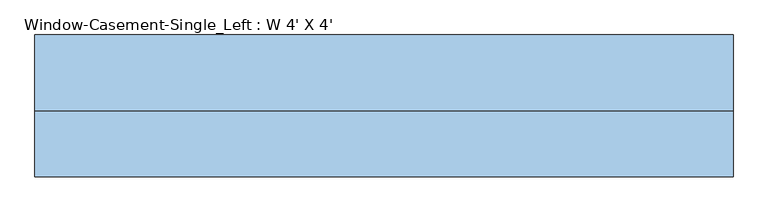
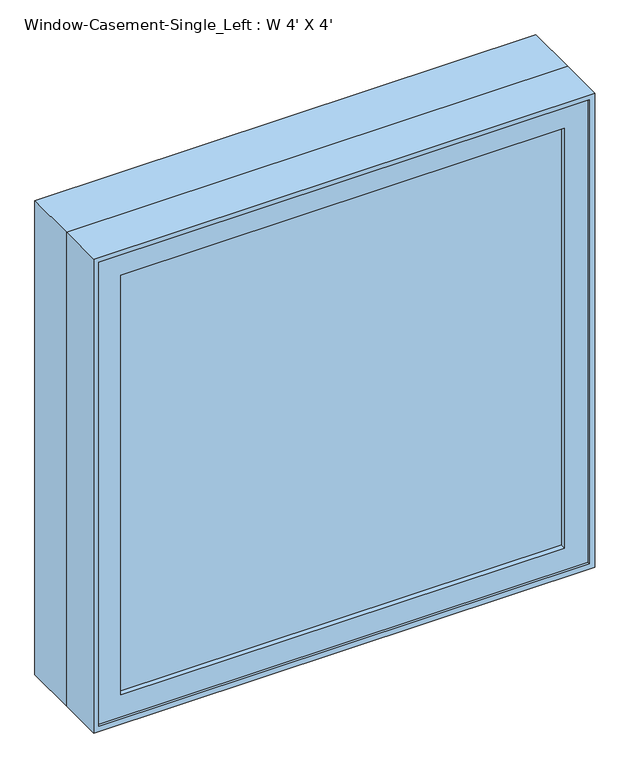
"""IFC4 building model written with IfcOpenShell, lengths in millimetres: window geometry, Window-Casement-Single_Left : W 4' X 4'."""

from ifc_helpers import new_model, si_unit, frame, origin, place, context, project, spatial, polyline, outline, extrude, faceted_brep, source, transform, mapped, element, save


def window_casement_single_left_w_4_x_4_e869003f(model_context):
    return source(origin(), model_context, "Body", "SolidModel", [
        faceted_brep([(577.85, -82.55, 2101.85), (-577.85, -82.55, 2101.85), (-577.85, -19.05, 2101.85), (577.85, -19.05, 2101.85), (596.9, -133.35, 2120.9), (-596.9, -133.35, 2120.9), (-596.9, -82.55, 2120.9), (596.9, -82.55, 2120.9), (609.6, -19.05, 2133.6), (-609.6, -19.05, 2133.6), (-609.6, -133.35, 2133.6), (609.6, -133.35, 2133.6), (-577.85, -82.55, 946.15), (-577.85, -19.05, 946.15), (-596.9, -133.35, 927.1), (-596.9, -82.55, 927.1), (-609.6, -19.05, 914.4), (-609.6, -133.35, 914.4), (577.85, -82.55, 946.15), (577.85, -19.05, 946.15), (596.9, -133.35, 927.1), (596.9, -82.55, 927.1), (609.6, -19.05, 914.4), (609.6, -133.35, 914.4)], [[[0, 1, 2, 3]], [[4, 5, 6, 7]], [[8, 9, 10, 11]], [[1, 12, 13, 2]], [[5, 14, 15, 6]], [[9, 16, 17, 10]], [[12, 18, 19, 13]], [[14, 20, 21, 15]], [[16, 22, 23, 17]], [[9, 8, 22, 16], [3, 2, 13, 19]], [[18, 0, 3, 19]], [[7, 6, 15, 21], [1, 0, 18, 12]], [[20, 4, 7, 21]], [[22, 8, 11, 23]], [[11, 10, 17, 23], [5, 4, 20, 14]]]),
        extrude(outline(polyline([(2133.6, -609.6), (914.4, -609.6), (914.4, 609.6), (2133.6, 609.6), (2133.6, -609.6)]), holes=[polyline([(2114.55, 590.55), (933.45, 590.55), (933.45, -590.55), (2114.55, -590.55), (2114.55, 590.55)])]), frame((0.0, -19.05, 0.0), z_axis=(0.0, 1.0, 0.0), x_axis=(0.0, 0.0, 1.0)), (0.0, 0.0, 1.0), 133.35),
        extrude(outline(polyline([(2120.9, 596.9), (2120.9, -596.9), (927.1, -596.9), (927.1, 596.9), (2120.9, 596.9)]), holes=[polyline([(2063.75, -539.75), (2063.75, 539.75), (984.25, 539.75), (984.25, -539.75), (2063.75, -539.75)])]), frame((0.0, -127.0, 0.0), z_axis=(0.0, 1.0, 0.0), x_axis=(0.0, 0.0, 1.0)), (0.0, 0.0, 1.0), 44.45),
        extrude(outline(polyline([(539.75, -114.3), (-539.75, -114.3), (-539.75, -107.95), (539.75, -107.95), (539.75, -114.3)])), frame((0.0, 0.0, 984.25), z_axis=(0.0, 0.0, 1.0), x_axis=(1.0, 0.0, 0.0)), (0.0, 0.0, 1.0), 1079.5),
        extrude(outline(polyline([(-539.75, -95.25), (539.75, -95.25), (539.75, -101.6), (-539.75, -101.6), (-539.75, -95.25)])), frame((0.0, 0.0, 984.25), z_axis=(0.0, 0.0, 1.0), x_axis=(1.0, 0.0, 0.0)), (0.0, 0.0, 1.0), 1079.5),
    ])


if __name__ == "__main__":
    model = new_model("IFC4")
    model_context = context("Model", 3, world=origin())
    ifc_project = project(units=[si_unit("LENGTHUNIT", "METRE", prefix="MILLI")], contexts=[model_context])
    site = spatial("IfcSite", under=ifc_project)
    building = spatial("IfcBuilding", under=site)
    placement = place(None, origin())
    window_casement_single_left_w_4_x_4_shape = window_casement_single_left_w_4_x_4_e869003f(model_context)
    element("IfcWindow", 1, ObjectType="Window-Casement-Single_Left : W 4' X 4'", at=placement, inside=building, context=model_context, shape_type="MappedRepresentation", body=[
        mapped(window_casement_single_left_w_4_x_4_shape, transform((0.0, 0.0, 0.0), x_axis=(1.0, 0.0, 0.0), y_axis=(0.0, 1.0, 0.0), z_axis=(0.0, 0.0, 1.0))),
    ])
    save(model, "model.ifc")

# Revit data of these elements
# Type "Window-Casement-Single_Left : W 4' X 4'"
#   Type Mark = "19"
#   Fire Rating = "0.5h"
#   Assembly Code = "B2020100"
#   Analytic Construction = "Double glazing - domestic"
#   Window Inset [instance default] = 0' - 0"
#   Wall Thickness [instance default] = 0' - 6"
#   Visual Light Transmittance = 0.81
#   Thermal Resistance (R) = 1.8146 (h·ft²·°F)/BTU
#   Solar Heat Gain Coefficient = 0.76
#   Rough Width = 4' - 0 1/2"
#   Rough Height = 4' - 0 1/2"
#   Interior Wall Closure [instance default] = 0' - 2 1/4"
#   Height = 4' - 0"
#   Heat Transfer Coefficient (U) = 0.5511 BTU/(h·ft²·°F)
#   Frame Extension [instance default] = 0' - 0 1/4"
#   Exterior Wall Closure [instance default] = 0' - 1 1/4"
#   Extension Jamb [instance default] = 0' - 2 1/4"
#   Default Sill Height = 3' - 0"
#   Width = 4' - 0"
#   Muntin Visibility = yes
#   Interior Trim Visibility [instance default] = yes
#   Exterior Trim Visibility [instance default] = yes
#   Extension Jamb Visibility [instance default] = yes
#   Muntin Pattern = Muntin Pattern_2x2 : Muntin Pattern_2x2
#   Interior Trim Material = Wood - Stained
#   Interior Trim = Trim-Window-Interior-Flat : Picture Frame
#   Interior Frame Material = Wood - Stained
#   Glass Panel Material = Glass
#   Exterior Trim Material = Clad - White
#   Exterior Trim = Trim-Window-Exterior-Flat : with Sill
#   Exterior Frame Material = Clad - White
#   Wall Closure = (empty or 0)
# Element 1 (IfcWindow, "Window-Casement-Single_Left : W 4' X 4'")
#   Wall Thickness = 0' - 9"
#   Extension Jamb = 0' - 5 1/4"
#   Materials on its faces: "Wood - Stained", "Glass", "Clad - White"
# Materials
#   "Wood - Stained": class "Wood", colour RGB 224 178 126, transparency 0, Cost = 0
#   "Glass": class "Glass", colour RGB 0 128 192, transparency 0.75, Description = "Soda Lime Glass", Cost = 0
#   "Clad - White": class "Wood", colour RGB 242 242 238, transparency 0, Cost = 0
